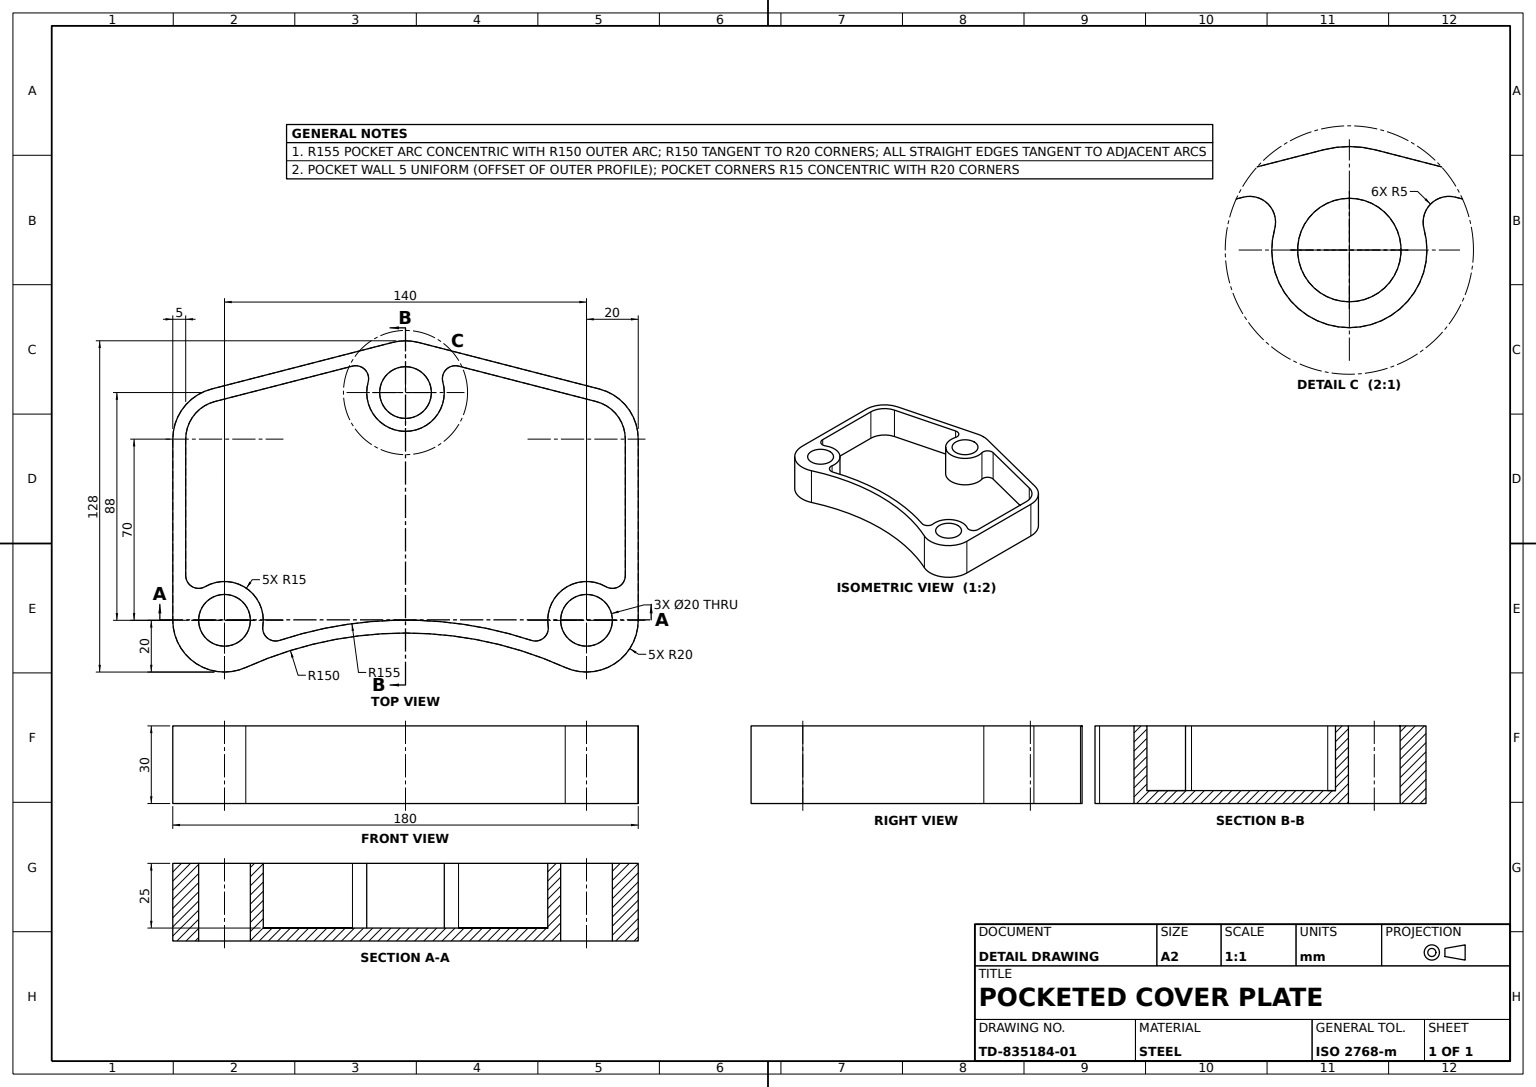
SolidWorks part; units mm, degrees
material "Plain Carbon Steel"
ref_plane "Front Plane" through (0, 0, 0) normal (0, 0, 1) x (1, 0, 0)
ref_plane "Top Plane" through (0, 0, 0) normal (0, 1, 0) x (1, 0, 0)
ref_plane "Right Plane" through (0, 0, 0) normal (1, 0, 0) x (0, 0, -1)
sketch "Base Plate Profile Sketch" plane through (0, 0, 0) normal (0, 1, 0) x (1, 0, 0)
  line L0 (0, -16.5) -> (0, 16.5) construction
  line L1 (-74.9808, 1.3699) -> (-4.9808, 19.3699)
  line L2 (74.9808, 1.3699) -> (4.9808, 19.3699)
  line L3 (-90, -18) -> (-90, -88)
  line L4 (90, -18) -> (90, -88)
  circle A1 centre (0, 0) radius 10
  arc A2 (4.9808, 19.3699) -> (-4.9808, 19.3699) centre (0, 0) ccw
  circle A3 centre (-70, -88) radius 10
  arc A5 (-90, -88) -> (-61.7647, -106.2258) centre (-70, -88) ccw
  circle A6 centre (70, -88) radius 10
  arc A8 (61.7647, -106.2258) -> (90, -88) centre (70, -88) ccw
  arc A9 (-74.9808, 1.3699) -> (-90, -18) centre (-70, -18) ccw
  arc A10 (74.9808, 1.3699) -> (90, -18) centre (70, -18) cw
  arc A11 (-61.7647, -106.2258) -> (61.7647, -106.2258) centre (0, -242.9193) cw
  dimension "D2" = 20
  dimension "D3" = 40
  dimension "D4" = 150
  dimension "D6" = 20
  dimension "D9" = 20
  dimension "D14" = 40
  dimension "D10" = 140
  dimension "D11" = 70
  dimension "D12" = 88
  dimension "D13" = 88
  dimension "D15" = 140
  dimension "D16" = 70
extrude "Base Plate 30mm" add sketch "Base Plate Profile Sketch" along normal blind 30 contours L3 A5 A11 A8 L4 A10 L2 A2 L1 A9
sketch "Pocket Profile Sketch" plane through (0, 30, 0) normal (0, 1, 0) x (1, 0, 0)
  line L2 (-85, -18) -> (-85, -88)
  line L3 (-85, -18) -> (-85, -70.6795)
  line L8 (-3.7356, 14.5274) -> (-73.7356, -3.4726)
  line L9 (-20.5104, 10.2139) -> (-73.7356, -3.4726)
  line L11 (73.7356, -3.4726) -> (3.7356, 14.5274)
  line L12 (73.7356, -3.4726) -> (20.5104, 10.2139)
  line L14 (85, -88) -> (85, -18)
  line L15 (85, -70.6795) -> (85, -18)
  arc A0 (-14.4489, 4.0286) -> (14.4489, 4.0286) centre (0, 0) ccw
  arc A1 (-55.1706, -90.2556) -> (-77.5, -75.0096) centre (-70, -88) ccw
  arc A2 (77.5, -75.0096) -> (55.1706, -90.2556) centre (70, -88) ccw
  arc A3 (-85, -70.6795) -> (-77.5, -75.0096) centre (-80, -70.6795) ccw
  arc A4 (77.5, -75.0096) -> (85, -70.6795) centre (80, -70.6795) ccw
  arc A5 (63.8235, -101.6694) -> (-63.8235, -101.6694) centre (0, -242.9193) ccw
  arc A6 (48.6578, -95.7547) -> (-48.6578, -95.7547) centre (0, -242.9193) ccw
  arc A7 (-55.1706, -90.2556) -> (-48.6578, -95.7547) centre (-50.2274, -91.0075) ccw
  arc A8 (48.6578, -95.7547) -> (55.1706, -90.2556) centre (50.2274, -91.0075) ccw
  arc A9 (-14.4489, 4.0286) -> (-20.5104, 10.2139) centre (-19.2652, 5.3714) ccw
  arc A10 (20.5104, 10.2139) -> (14.4489, 4.0286) centre (19.2652, 5.3714) ccw
  arc A12 (-73.7356, -3.4726) -> (-85, -18) centre (-70, -18) ccw
  arc A13 (-73.7356, -3.4726) -> (-85, -18) centre (-70, -18) ccw
  arc A15 (85, -18) -> (73.7356, -3.4726) centre (70, -18) ccw
  arc A16 (85, -18) -> (73.7356, -3.4726) centre (70, -18) ccw
  dimension "D1" = 30
  dimension "D2" = 30
  dimension "D3" = 30
  dimension "D10" = 10
  dimension "D11" = 10
  dimension "D12" = 10
  dimension "D13" = 10
  dimension "D14" = 10
  dimension "D15" = 10
  dimension "D4" = 5
  dimension "D5" = 5
  dimension "D6" = 5
  dimension "D7" = 5
  dimension "D8" = 5
  dimension "D9" = 5
extrude "Pocket 25mm Deep" cut sketch "Pocket Profile Sketch" against normal blind 25
